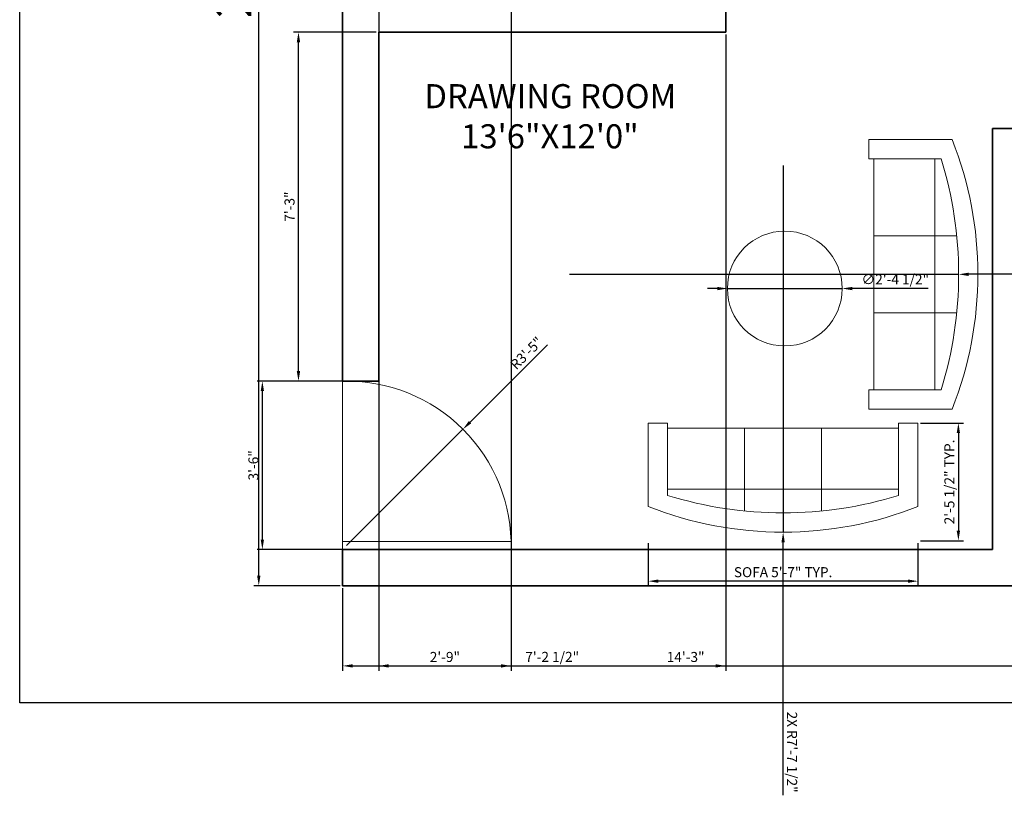
# Model space of a CAD drawing. Units: inches. Extents: x 5717 to 6221, y 11359 to 11763.
# Tile 1 of 4: x 5717 to 5963, y 11359 to 11552. Entities that reach past the tile are written whole.
import ezdxf

# ---------------------------------------------------------------- set-up
doc = ezdxf.new("R2010")
doc.units = ezdxf.units.IN
for name, color, linetype, lineweight, true_color in [('A-ANNO-DIMS', 254, 'Continuous', 13, 0xfeeab9), ('A-ANNO-TTLB', 51, 'Continuous', 25, 0xf8f6b0), ('A-AREA-IDEN', 11, 'Continuous', 20, 0xf27172), ('A-WALL', 244, 'Continuous', 35, 0x991b1e)]:
    doc.layers.add(name, color=color, linetype=linetype, lineweight=lineweight, true_color=true_color)
doc.layers.add('A-DOOR', color=5, linetype='Continuous', lineweight=18)
doc.layers.add('A-FURN', color=8, linetype='Continuous', lineweight=18)
doc.styles.get("Standard").update_dxf_attribs({"font": 'arial.ttf'})
doc.dimstyles.new('ISO-25', dxfattribs={"dimtxt": 2.5, "dimasz": 2.5, "dimexe": 1.25, "dimexo": 0.625, "dimtad": 1, "dimlunit": 3, "dimtxsty": 'Standard', "dimcen": 2.5, "dimadec": 0, "dimazin": 0, "dimtfac": 1, "dimtmove": 0, "dimatfit": 3, "dimfxl": 1, "dimarcsym": 0})

# ---------------------------------------------------------------- blocks, each defined once
blk = doc.blocks.new('*D13')
at = {"layer": 'A-ANNO-DIMS', "color": 0, "lineweight": -2, "transparency": 16777216}
for p, q in [((5797.28, 11711.11), (5775.76, 11711.11)), ((5777.01, 11413.61), (5777.01, 11708.61)), ((5797.28, 11411.11), (5775.76, 11411.11))]:
    blk.add_line(p, q, dxfattribs=at)
at = {"layer": 'A-ANNO-DIMS', "color": 0, "transparency": 16777216}
for points in [[(5776.6, 11708.61), (5777.43, 11708.61), (5777.01, 11711.11)], [(5776.6, 11413.61), (5777.43, 11413.61), (5777.01, 11411.11)]]:
    blk.add_solid(points, dxfattribs=at)
at = {"layer": 'Defpoints', "color": 0, "transparency": 16777216}
for p in [(5777.01, 11711.11), (5797.9, 11711.11), (5797.9, 11411.11)]:
    blk.add_point(p, dxfattribs=at)
at = {"layer": 'A-ANNO-DIMS', "color": 0, "transparency": 16777216, "insert": (5771.79, 11561.11), "char_height": 9, "attachment_point": 5, "rotation": 90}
blk.add_mtext("25'", dxfattribs=at)
blk = doc.blocks.new('Sofa - Roundback 7 ft.')
for p, q in [((-12.00002, -32.4421), (-12.00003, -6.5971)), ((11.99997, -32.4421), (11.99998, -6.5971)), ((-36.000027, -34), (-36.000027, -11.4696)), ((35.99998, -34), (35.99998, -11.4696)), ((-35.999844, -13.3819), (35.9998, -13.3819)), ((-36.000027, -32.4421), (35.99998, -32.4421))]:
    blk.add_line(p, q)
for points in [[(-36.000027, -34), (-42.000027, -34), (-42.000027, -8)], [(41.99998, -8), (41.99998, -34), (35.99998, -34)]]:
    blk.add_lwpolyline(points)
for centre, radius, start, end in [((0, -114.25), 114.25, 68.43141, 111.5686), ((-0.00001, -127.1968), 121.1968, 72.72033, 107.2797)]:
    blk.add_arc(centre, radius, start, end)
blk = doc.blocks.new('*D22')
at = {"layer": 'A-ANNO-DIMS', "color": 0, "lineweight": -2, "transparency": 16777216}
for p, q in [((5874.1, 11421.69), (5874.1, 11410.98)), ((5941.3, 11421.69), (5941.3, 11410.98)), ((5938.8, 11412.23), (5876.6, 11412.23))]:
    blk.add_line(p, q, dxfattribs=at)
at = {"layer": 'A-ANNO-DIMS', "color": 0, "transparency": 16777216}
for points in [[(5876.6, 11412.65), (5876.6, 11411.82), (5874.1, 11412.23)], [(5938.8, 11412.65), (5938.8, 11411.82), (5941.3, 11412.23)]]:
    blk.add_solid(points, dxfattribs=at)
at = {"layer": 'Defpoints', "color": 0, "transparency": 16777216}
for p in [(5874.1, 11422.31), (5941.3, 11422.31), (5874.1, 11412.23)]:
    blk.add_point(p, dxfattribs=at)
at = {"layer": 'A-ANNO-DIMS', "color": 0, "transparency": 16777216, "insert": (5907.7, 11414.15), "char_height": 2.5, "attachment_point": 5}
blk.add_mtext('SOFA 5\'-7" TYP.', dxfattribs=at)
blk = doc.blocks.new('*D23')
at = {"layer": 'A-ANNO-DIMS', "color": 0, "lineweight": -2, "transparency": 16777216}
for p, q in [((5941.92, 11451.65), (5952.63, 11451.65)), ((5951.38, 11449.15), (5951.38, 11424.81)), ((5941.92, 11422.31), (5952.63, 11422.31))]:
    blk.add_line(p, q, dxfattribs=at)
at = {"layer": 'A-ANNO-DIMS', "color": 0, "transparency": 16777216}
for points in [[(5950.96, 11449.15), (5951.79, 11449.15), (5951.38, 11451.65)], [(5950.96, 11424.81), (5951.79, 11424.81), (5951.38, 11422.31)]]:
    blk.add_solid(points, dxfattribs=at)
at = {"layer": 'Defpoints', "color": 0, "transparency": 16777216}
for p in [(5941.3, 11451.65), (5941.3, 11422.31), (5951.38, 11422.31)]:
    blk.add_point(p, dxfattribs=at)
at = {"layer": 'A-ANNO-DIMS', "color": 0, "transparency": 16777216, "insert": (5949.46, 11436.98), "char_height": 2.5, "attachment_point": 5, "rotation": 90}
blk.add_mtext('2\'-5 1/2" TYP.', dxfattribs=at)
blk = doc.blocks.new('*D38')
at = {"layer": 'A-ANNO-DIMS', "color": 0, "lineweight": -2, "transparency": 16777216}
for p, q in [((5797.9, 11410.48), (5797.9, 11389.86)), ((5968.9, 11410.48), (5968.9, 11389.86)), ((5800.4, 11391.11), (5966.4, 11391.11))]:
    blk.add_line(p, q, dxfattribs=at)
at = {"layer": 'A-ANNO-DIMS', "color": 0, "transparency": 16777216}
for points in [[(5800.4, 11391.53), (5800.4, 11390.69), (5797.9, 11391.11)], [(5966.4, 11391.53), (5966.4, 11390.69), (5968.9, 11391.11)]]:
    blk.add_solid(points, dxfattribs=at)
at = {"layer": 'Defpoints', "color": 0, "transparency": 16777216}
for p in [(5797.9, 11411.11), (5968.9, 11411.11), (5968.9, 11391.11)]:
    blk.add_point(p, dxfattribs=at)
at = {"layer": 'A-ANNO-DIMS', "color": 0, "transparency": 16777216, "insert": (5883.4, 11393.01), "char_height": 2.5, "attachment_point": 5}
blk.add_mtext('14\'-3"', dxfattribs=at)
blk = doc.blocks.new('*D47')
at = {"layer": 'A-ANNO-DIMS', "color": 0, "lineweight": -2, "transparency": 16777216}
for p, q in [((5806.28, 11462.11), (5776.65, 11462.11)), ((5777.9, 11422.61), (5777.9, 11459.61)), ((5839.28, 11420.11), (5776.65, 11420.11))]:
    blk.add_line(p, q, dxfattribs=at)
at = {"layer": 'A-ANNO-DIMS', "color": 0, "transparency": 16777216}
for points in [[(5777.49, 11459.61), (5778.32, 11459.61), (5777.9, 11462.11)], [(5777.49, 11422.61), (5778.32, 11422.61), (5777.9, 11420.11)]]:
    blk.add_solid(points, dxfattribs=at)
at = {"layer": 'Defpoints', "color": 0, "transparency": 16777216}
for p in [(5777.9, 11462.11), (5806.9, 11462.11), (5839.9, 11420.11)]:
    blk.add_point(p, dxfattribs=at)
at = {"layer": 'A-ANNO-DIMS', "color": 0, "transparency": 16777216, "insert": (5776, 11441.11), "char_height": 2.5, "attachment_point": 5, "rotation": 90}
blk.add_mtext('3\'-6"', dxfattribs=at)
blk = doc.blocks.new('*D48')
at = {"layer": 'A-ANNO-DIMS', "color": 0, "lineweight": -2, "transparency": 16777216}
for p, q in [((5806.28, 11549.11), (5785.65, 11549.11)), ((5786.9, 11464.61), (5786.9, 11546.61)), ((5806.28, 11462.11), (5785.65, 11462.11))]:
    blk.add_line(p, q, dxfattribs=at)
at = {"layer": 'A-ANNO-DIMS', "color": 0, "transparency": 16777216}
for points in [[(5786.49, 11546.61), (5787.32, 11546.61), (5786.9, 11549.11)], [(5786.49, 11464.61), (5787.32, 11464.61), (5786.9, 11462.11)]]:
    blk.add_solid(points, dxfattribs=at)
at = {"layer": 'Defpoints', "color": 0, "transparency": 16777216}
for p in [(5786.9, 11549.11), (5806.9, 11549.11), (5806.9, 11462.11)]:
    blk.add_point(p, dxfattribs=at)
at = {"layer": 'A-ANNO-DIMS', "color": 0, "transparency": 16777216, "insert": (5785, 11505.61), "char_height": 2.5, "attachment_point": 5, "rotation": 90}
blk.add_mtext('7\'-3"', dxfattribs=at)
blk = doc.blocks.new('*D55')
at = {"layer": 'A-ANNO-DIMS', "color": 0, "lineweight": -2, "transparency": 16777216}
for p, q in [((5806.9, 11548.48), (5806.9, 11389.86)), ((5893.38, 11548.48), (5893.38, 11389.86)), ((5809.4, 11391.11), (5890.88, 11391.11))]:
    blk.add_line(p, q, dxfattribs=at)
at = {"layer": 'A-ANNO-DIMS', "color": 0, "transparency": 16777216}
for points in [[(5809.4, 11391.53), (5809.4, 11390.69), (5806.9, 11391.11)], [(5890.88, 11391.53), (5890.88, 11390.69), (5893.38, 11391.11)]]:
    blk.add_solid(points, dxfattribs=at)
at = {"layer": 'Defpoints', "color": 0, "transparency": 16777216}
for p in [(5806.9, 11549.11), (5893.38, 11549.11), (5893.38, 11391.11)]:
    blk.add_point(p, dxfattribs=at)
at = {"layer": 'A-ANNO-DIMS', "color": 0, "transparency": 16777216, "insert": (5850.14, 11393.03), "char_height": 2.5, "attachment_point": 5}
blk.add_mtext('7\'-2 1/2"', dxfattribs=at)
blk = doc.blocks.new('*D56')
at = {"layer": 'A-ANNO-DIMS', "color": 0, "lineweight": -2, "transparency": 16777216}
for p, q in [((5806.9, 11659.48), (5806.9, 11389.86)), ((5839.9, 11659.48), (5839.9, 11389.86)), ((5809.4, 11391.11), (5837.4, 11391.11))]:
    blk.add_line(p, q, dxfattribs=at)
at = {"layer": 'A-ANNO-DIMS', "color": 0, "transparency": 16777216}
for points in [[(5809.4, 11391.53), (5809.4, 11390.69), (5806.9, 11391.11)], [(5837.4, 11391.53), (5837.4, 11390.69), (5839.9, 11391.11)]]:
    blk.add_solid(points, dxfattribs=at)
at = {"layer": 'Defpoints', "color": 0, "transparency": 16777216}
for p in [(5806.9, 11660.11), (5839.9, 11660.11), (5839.9, 11391.11)]:
    blk.add_point(p, dxfattribs=at)
at = {"layer": 'A-ANNO-DIMS', "color": 0, "transparency": 16777216, "insert": (5823.4, 11393.01), "char_height": 2.5, "attachment_point": 5}
blk.add_mtext('2\'-9"', dxfattribs=at)
blk = doc.blocks.new('*D58')
at = {"layer": 'A-ANNO-DIMS', "color": 0, "lineweight": -2, "transparency": 16777216}
for p, q in [((5891.31, 11485.19), (5888.81, 11485.19)), ((5893.81, 11485.19), (5922.43, 11485.19)), ((5943.87, 11485.19), (5924.93, 11485.19))]:
    blk.add_line(p, q, dxfattribs=at)
at = {"layer": 'A-ANNO-DIMS', "color": 0, "transparency": 16777216}
for points in [[(5891.31, 11485.6), (5891.31, 11484.77), (5893.81, 11485.19)], [(5924.93, 11485.6), (5924.93, 11484.77), (5922.43, 11485.19)]]:
    blk.add_solid(points, dxfattribs=at)
at = {"layer": 'Defpoints', "color": 0, "transparency": 16777216}
for p in [(5893.81, 11485.19), (5922.43, 11485.19)]:
    blk.add_point(p, dxfattribs=at)
at = {"layer": 'A-ANNO-DIMS', "color": 0, "transparency": 16777216, "insert": (5935.65, 11487.16), "char_height": 2.5, "attachment_point": 5, "rotation": 359.9983}
blk.add_mtext('∅2\'-4 1/2"', dxfattribs=at)
blk = doc.blocks.new('*D59')
at = {"layer": 'A-ANNO-DIMS', "color": 0, "lineweight": -2, "transparency": 16777216}
for p, q in [((5848.94, 11471.15), (5829.67, 11451.88)), ((5798.9, 11421.11), (5827.9, 11450.11))]:
    blk.add_line(p, q, dxfattribs=at)
at = {"layer": 'A-ANNO-DIMS', "color": 0, "transparency": 16777216}
blk.add_solid([(5829.38, 11452.17), (5829.96, 11451.58), (5827.9, 11450.11)], dxfattribs=at)
at = {"layer": 'Defpoints', "color": 0, "transparency": 16777216}
for p in [(5827.9, 11450.11), (5798.9, 11421.11)]:
    blk.add_point(p, dxfattribs=at)
at = {"layer": 'A-ANNO-DIMS', "color": 0, "transparency": 16777216, "insert": (5843.96, 11468.85), "char_height": 2.5, "attachment_point": 5, "rotation": 45.0005}
blk.add_mtext('R3\'-5"', dxfattribs=at)
blk = doc.blocks.new('*D67')
at = {"layer": 'A-ANNO-DIMS', "color": 0, "lineweight": -2, "transparency": 16777216}
for p, q in [((5854.49, 11488.73), (5951.44, 11488.73)), ((6017.47, 11488.73), (5953.94, 11488.73))]:
    blk.add_line(p, q, dxfattribs=at)
at = {"layer": 'A-ANNO-DIMS', "color": 0, "transparency": 16777216}
blk.add_solid([(5953.94, 11489.15), (5953.94, 11488.32), (5951.44, 11488.73)], dxfattribs=at)
at = {"layer": 'Defpoints', "color": 0, "transparency": 16777216}
for p in [(5854.49, 11488.73), (5951.44, 11488.73)]:
    blk.add_point(p, dxfattribs=at)
at = {"layer": 'A-ANNO-DIMS', "color": 0, "transparency": 16777216, "insert": (6009.62, 11490.64), "char_height": 2.5, "attachment_point": 5, "rotation": 360}
blk.add_mtext('2X R8\'-1"', dxfattribs=at)
blk = doc.blocks.new('*D68')
at = {"layer": 'A-ANNO-DIMS', "color": 0, "lineweight": -2, "transparency": 16777216}
for p, q in [((5907.7, 11515.85), (5907.7, 11424.45)), ((5907.7, 11358.84), (5907.7, 11421.95))]:
    blk.add_line(p, q, dxfattribs=at)
at = {"layer": 'A-ANNO-DIMS', "color": 0, "transparency": 16777216}
blk.add_solid([(5908.11, 11421.95), (5907.28, 11421.95), (5907.7, 11424.45)], dxfattribs=at)
at = {"layer": 'Defpoints', "color": 0, "transparency": 16777216}
for p in [(5907.7, 11515.85), (5907.7, 11424.45)]:
    blk.add_point(p, dxfattribs=at)
at = {"layer": 'A-ANNO-DIMS', "color": 0, "transparency": 16777216, "insert": (5909.61, 11369.61), "char_height": 2.5, "attachment_point": 5, "rotation": 270.0002}
blk.add_mtext('2X R7\'-7 1/2"', dxfattribs=at)

msp = doc.modelspace()

# ---------------------------------------------------------------- linework, layer by layer
at = {"layer": 'A-ANNO-TTLB'}
msp.add_lwpolyline([(5717.423, 11763.126), (6221.432, 11763.126), (6221.432, 11381.867), (5717.423, 11381.867)], close=True, dxfattribs=at)
at = {"layer": 'A-DOOR'}
for p, q in [((5797.902, 11420.109), (5797.902, 11462.109)), ((5797.902, 11462.109), (5797.902, 11420.109)), ((5839.902, 11422.109), (5797.902, 11422.109)), ((5839.902, 11420.109), (5839.902, 11422.109)), ((5797.902, 11420.109), (5839.902, 11420.109))]:
    msp.add_line(p, q, dxfattribs=at)
msp.add_arc((5798.902, 11421.109), 41.012, 358.60282, 91.39718, dxfattribs=at)
at = {"layer": 'A-FURN'}
msp.add_circle((5908.12, 11485.186), 14.31, dxfattribs=at)
at = {"layer": 'A-WALL'}
for p, q in [((5797.902, 11711.109), (5797.902, 11462.109)), ((5893.38, 11558.109), (5893.38, 11549.109)), ((5873.902, 11549.109), (5806.902, 11549.109)), ((5806.902, 11549.109), (5806.902, 11462.109)), ((5893.38, 11549.109), (5873.902, 11549.109)), ((5959.902, 11420.109), (5959.902, 11525.109)), ((5959.902, 11525.109), (5968.902, 11525.109)), ((5797.902, 11462.109), (5806.902, 11462.109)), ((5797.902, 11420.109), (5959.902, 11420.109)), ((5797.902, 11420.109), (5797.902, 11411.109)), ((5797.902, 11411.109), (6157.902, 11411.109))]:
    msp.add_line(p, q, dxfattribs=at)

# ---------------------------------------------------------------- block references
at = {"layer": 'A-FURN', "xscale": 0.8, "yscale": 0.8, "zscale": 0.8}
for p, rotation in [((5956.243, 11488.735), 270), ((5907.696, 11424.447), 180)]:
    msp.add_blockref('Sofa - Roundback 7 ft.', p, dxfattribs=dict(at, rotation=rotation))

# ---------------------------------------------------------------- texts
at = {"layer": 'A-AREA-IDEN', "insert": (5816.45, 11536.146), "char_height": 6, "attachment_point": 1}
msp.add_mtext_dynamic_manual_height_columns(' DRAWING ROOM\\P      13\'6"X12\'0"', width=116.60264, gutter_width=12.5, heights=[0], dxfattribs=at)

# ---------------------------------------------------------------- dimensions: what is measured, and where the dimension line sits
at = {"layer": 'A-ANNO-DIMS'}
for base, p1, p2, override, picture, middle in [((5777.014, 11711.109), (5797.902, 11411.109), (5797.902, 11711.109), {"dimtxt": 9, "dimclrd": 0, "dimclre": 0, "dimclrt": 0}, '*D13', (5771.794, 11561.109)), ((5786.902, 11549.109), (5806.902, 11462.109), (5806.902, 11549.109), {"dimdec": 1, "dimlfac": 1, "dimrnd": 0, "dimzin": 1, "dimdsep": 46, "dimlunit": 4, "dimfrac": 2}, '*D48', (5785, 11505.609)), ((5777.902, 11462.109), (5839.902, 11420.109), (5806.902, 11462.109), {"dimdec": 1, "dimlfac": 1, "dimrnd": 0, "dimzin": 1, "dimdsep": 46, "dimlunit": 4, "dimfrac": 2}, '*D47', (5776, 11441.109))]:
    dim = msp.add_linear_dim(base=base, p1=p1, p2=p2, angle=90, dimstyle='ISO-25', override=override, dxfattribs=at)
    dim.commit()
    dim.dimension.update_dxf_attribs({"geometry": picture, "text_midpoint": middle})
for base, p1, p2, picture, middle in [((5839.905, 11391.109), (5806.902, 11660.109), (5839.905, 11660.109), '*D56', (5823.404, 11393.01)), ((5893.38, 11391.109), (5806.902, 11549.109), (5893.38, 11549.109), '*D55', (5850.141, 11393.026)), ((5968.902, 11391.109), (5797.902, 11411.109), (5968.902, 11411.109), '*D38', (5883.402, 11393.011))]:
    dim = msp.add_linear_dim(base=base, p1=p1, p2=p2, dimstyle='ISO-25', override={"dimdec": 1, "dimlfac": 1, "dimrnd": 0, "dimzin": 1, "dimdsep": 46, "dimlunit": 4, "dimfrac": 2}, dxfattribs=at)
    dim.commit()
    dim.dimension.update_dxf_attribs({"geometry": picture, "text_midpoint": middle})
for center, mpoint, picture, middle in [((5907.696, 11515.847), (5907.696, 11424.447), '*D68', (5907.696, 11369.607)), ((5854.485, 11488.735), (5951.443, 11488.735), '*D67', (6009.617, 11488.735))]:
    dim = msp.add_radius_dim(center=center, mpoint=mpoint, text='2X <>', dimstyle='ISO-25', override={"dimdec": 1, "dimlfac": 1, "dimrnd": 0, "dimzin": 1, "dimdsep": 46, "dimlunit": 4, "dimfrac": 2}, dxfattribs=at)
    dim.commit()
    dim.dimension.update_dxf_attribs({"geometry": picture, "text_midpoint": middle, "dimtype": 164})
dim = msp.add_diameter_dim_2p(p1=(5893.811, 11485.187), p2=(5922.43, 11485.186), dimstyle='ISO-25', override={"dimdec": 1, "dimlfac": 1, "dimrnd": 0, "dimzin": 1, "dimdsep": 46, "dimlunit": 4, "dimfrac": 2}, dxfattribs=at)
dim.commit()
dim.dimension.update_dxf_attribs({"geometry": '*D58', "text_midpoint": (5935.651, 11485.186), "dimtype": 163})
dim = msp.add_radius_dim(center=(5798.902, 11421.109), mpoint=(5827.902, 11450.109), dimstyle='ISO-25', override={"dimdec": 1, "dimlfac": 1, "dimrnd": 0, "dimzin": 1, "dimdsep": 46, "dimlunit": 4, "dimfrac": 2}, dxfattribs=at)
dim.commit()
dim.dimension.update_dxf_attribs({"geometry": '*D59', "text_midpoint": (5845.302, 11467.509), "dimtype": 164})
for base, p1, p2, angle, text, picture, middle in [((5951.376, 11422.314), (5941.296, 11451.647), (5941.296, 11422.314), 270, '<> TYP.', '*D23', (5949.458, 11436.98)), ((5874.096, 11412.234), (5941.296, 11422.314), (5874.096, 11422.314), 180, 'SOFA <> TYP.', '*D22', (5907.696, 11414.152))]:
    dim = msp.add_linear_dim(base=base, p1=p1, p2=p2, angle=angle, text=text, dimstyle='ISO-25', override={"dimdec": 1, "dimlfac": 1, "dimrnd": 0, "dimzin": 1, "dimdsep": 46, "dimlunit": 4, "dimfrac": 2}, dxfattribs=at)
    dim.commit()
    dim.dimension.update_dxf_attribs({"geometry": picture, "text_midpoint": middle})

doc.saveas('drawing.dxf')
